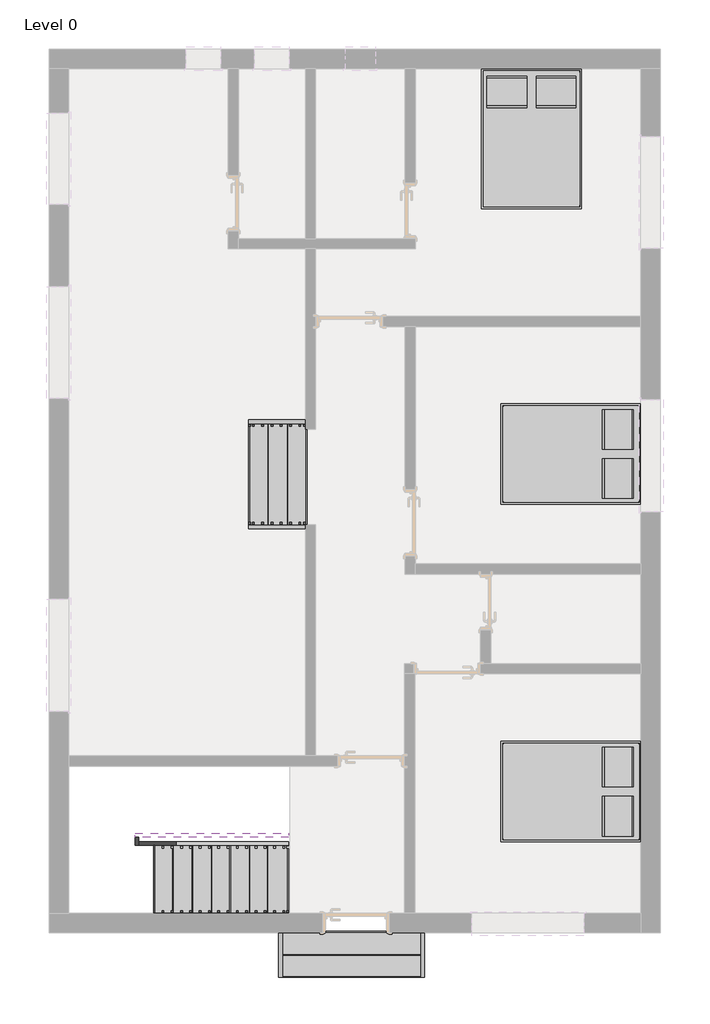
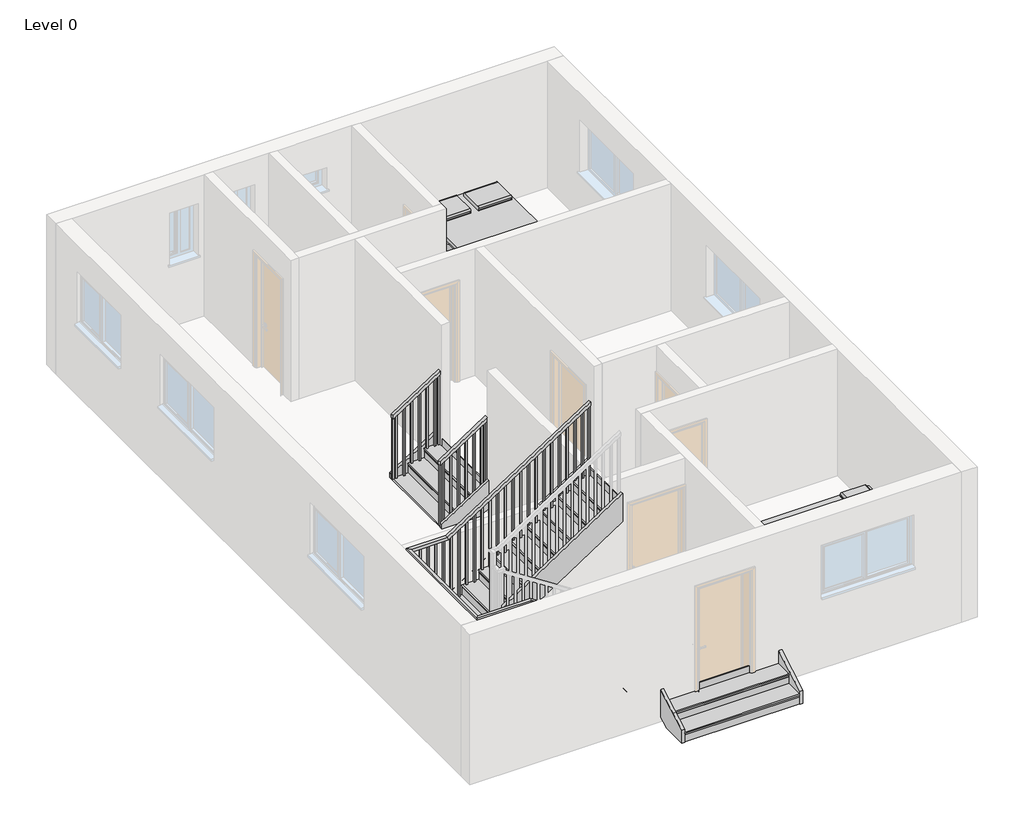
# One storey, part 2 of 2: 10 members, 3 furniture elements, 3 railings, 3 stair flights.
"""IFC4 building model written with IfcOpenShell, lengths in millimetres."""

from ifc_helpers import new_model, si_unit, frame, origin, place, context, project, spatial, polyline, outline, extrude, faceted_brep, transform, mapped, element, save
from components import furniture_bed_1_1346x1880x355mm_double_93dec6ea, wood_steps_w_50mm_tread_10mm_nosing_13mm_riser_0e3a26d2, wood_steps_w_50mm_tread_10mm_nosing_13mm_riser_e56a5079, wood_steps_w_50mm_tread_10mm_nosing_13mm_riser_d55d0cb6

model = new_model("IFC4")

# Units and contexts
model_context = context("Model", 3, world=origin())
ifc_project = project(units=[si_unit("LENGTHUNIT", "METRE", prefix="MILLI")], contexts=[model_context])

# Site, building, storey
site = spatial("IfcSite", under=ifc_project)
building = spatial("IfcBuilding", under=site)
storey = spatial("IfcBuildingStorey", under=building, Name="Level 0", Elevation=0.0)

# Furniture
placement = place(None, origin())
furniture_bed_1_1346x1880x355mm_double_shape = furniture_bed_1_1346x1880x355mm_double_93dec6ea(model_context)
element("IfcFurniture", 1, ObjectType="Furniture_Bed_1 : 1346x1880x355mm-Double", at=placement, inside=storey, context=model_context, shape_type="MappedRepresentation", body=[
    mapped(furniture_bed_1_1346x1880x355mm_double_shape, transform((-1450.4609005, 2546.998858, 400.0), x_axis=(0.0, -1.0, 0.0), y_axis=(1.0, 0.0, 0.0), z_axis=(0.0, 0.0, 1.0))),
])
element("IfcFurniture", 2, ObjectType="Furniture_Bed_1 : 1346x1880x355mm-Double", at=placement, inside=storey, context=model_context, shape_type="MappedRepresentation", body=[
    mapped(furniture_bed_1_1346x1880x355mm_double_shape, transform((-1450.4609005, 7079.151317, 400.0), x_axis=(0.0, -1.0, 0.0), y_axis=(1.0, 0.0, 0.0), z_axis=(0.0, 0.0, 1.0))),
])
element("IfcFurniture", 3, ObjectType="Furniture_Bed_1 : 1346x1880x355mm-Double", at=placement, inside=storey, context=model_context, shape_type="MappedRepresentation", body=[
    mapped(furniture_bed_1_1346x1880x355mm_double_shape, transform((-2557.0428677, 11207.1937668, 400.0), x_axis=(1.0, 0.0, 0.0), y_axis=(0.0, 1.0, 0.0), z_axis=(0.0, 0.0, 1.0))),
])

# Members
element("IfcMember", 4, ObjectType="Stringer-50mm_Width", at=placement, inside=storey, context=model_context, shape_type="SweptSolid", body=[
    extrude(outline(polyline([(230.7827164, -6016.6079187), (0.0, -6016.6079187), (0.0, -5634.3345887), (241.6372396, -5254.8904087), (715.8588519, -5254.8904087), (230.7827164, -6016.6079187)])), frame((0.0, 7148.1063074, 0.0), z_axis=(0.0, 1.0, 0.0), x_axis=(0.0, 0.0, 1.0)), (0.0, 0.0, 1.0), 50.0),
])
element("IfcMember", 5, ObjectType="Stringer-50mm_Width", at=placement, inside=storey, context=model_context, shape_type="SweptSolid", body=[
    extrude(outline(polyline([(230.7827164, -6016.6079187), (0.0, -6016.6079187), (0.0, -5634.3345887), (241.6372396, -5254.8904087), (715.8588519, -5254.8904087), (230.7827164, -6016.6079187)])), frame((0.0, 5736.998858, 0.0), z_axis=(0.0, 1.0, 0.0), x_axis=(0.0, 0.0, 1.0)), (0.0, 0.0, 1.0), 50.0),
])
element("IfcMember", 6, ObjectType="Stringer-50mm_Width", at=placement, inside=storey, context=model_context, shape_type="SweptSolid", body=[
    extrude(outline(polyline([(-287.2357414, 0.0), (-287.2357414, 221.2018083), (312.7642586, 554.5351417), (312.7642586, 96.9515798), (138.2514149, 0.0), (-287.2357414, 0.0)])), frame((-5613.3767794, 0.0, 0.0), z_axis=(1.0, 0.0, 0.0), x_axis=(0.0, 1.0, 0.0)), (0.0, 0.0, 1.0), 50.0),
])
element("IfcMember", 7, ObjectType="Stringer-50mm_Width", at=placement, inside=storey, context=model_context, shape_type="SweptSolid", body=[
    extrude(outline(polyline([(-287.2357414, 0.0), (-287.2357414, 221.2018083), (312.7642586, 554.5351417), (312.7642586, 96.9515798), (138.2514149, 0.0), (-287.2357414, 0.0)])), frame((-3703.3767794, 0.0, 0.0), z_axis=(1.0, 0.0, 0.0), x_axis=(0.0, 1.0, 0.0)), (0.0, 0.0, 1.0), 50.0),
])
element("IfcMember", 8, ObjectType="Stringer-50mm_Width", at=placement, inside=storey, context=model_context, shape_type="SweptSolid", body=[
    extrude(outline(polyline([(0.0, -5481.4951322), (214.9211649, -5481.4951322), (1542.4365081, -7506.9042559), (1542.4365081, -8236.5950487), (0.0, -5883.2776334), (0.0, -5481.4951322)])), frame((0.0, 522.7642586, 0.0), z_axis=(0.0, 1.0, 0.0), x_axis=(0.0, 0.0, 1.0)), (0.0, 0.0, 1.0), 50.0),
])
element("IfcMember", 9, ObjectType="Stringer-50mm_Width", at=placement, inside=storey, context=model_context, shape_type="SweptSolid", body=[
    extrude(outline(polyline([(-8434.8904087, 522.7642586), (-8484.8904087, 522.7642586), (-8484.8904087, 2546.998858), (-8434.8904087, 2546.998858), (-8434.8904087, 522.7642586)])), frame((0.0, 0.0, 1142.4365081), z_axis=(0.0, 0.0, 1.0), x_axis=(1.0, 0.0, 0.0)), (0.0, 0.0, 1.0), 400.0),
])
element("IfcMember", 10, ObjectType="Stringer-50mm_Width", at=placement, inside=storey, context=model_context, shape_type="SweptSolid", body=[
    extrude(outline(polyline([(1142.4365081, -7710.9666442), (2603.7006078, -5481.4951322), (3081.9623634, -5481.4951322), (1142.4365081, -8440.657437), (1142.4365081, -7710.9666442)])), frame((0.0, 2546.998858, 0.0), z_axis=(0.0, 1.0, 0.0), x_axis=(0.0, 0.0, 1.0)), (0.0, 0.0, 1.0), 50.0),
])
element("IfcMember", 11, ObjectType="Stringer-50mm_Width", at=placement, inside=storey, context=model_context, shape_type="SweptSolid", body=[
    extrude(outline(polyline([(0.0, -5481.4951322), (214.9211649, -5481.4951322), (1532.3368952, -7491.4951322), (1054.0751396, -7491.4951322), (0.0, -5883.2776334), (0.0, -5481.4951322)])), frame((0.0, 1486.5182736, 0.0), z_axis=(0.0, 1.0, 0.0), x_axis=(0.0, 0.0, 1.0)), (0.0, 0.0, 1.0), 50.0),
])
element("IfcMember", 12, ObjectType="Stringer-50mm_Width", at=placement, inside=storey, context=model_context, shape_type="SweptSolid", body=[
    extrude(outline(polyline([(-7491.4951322, 1486.5182736), (-7541.4951322, 1486.5182736), (-7541.4951322, 1596.5182736), (-7491.4951322, 1596.5182736), (-7491.4951322, 1486.5182736)])), frame((0.0, 0.0, 1142.4365081), z_axis=(0.0, 0.0, 1.0), x_axis=(1.0, 0.0, 0.0)), (0.0, 0.0, 1.0), 400.0),
])
element("IfcMember", 13, ObjectType="Stringer-50mm_Width", at=placement, inside=storey, context=model_context, shape_type="SweptSolid", body=[
    extrude(outline(polyline([(1731.7750974, -7541.4951322), (1253.5133419, -7541.4951322), (2603.7006078, -5481.4951322), (3081.9623634, -5481.4951322), (1731.7750974, -7541.4951322)])), frame((0.0, 1596.5182736, 0.0), z_axis=(0.0, 1.0, 0.0), x_axis=(0.0, 0.0, 1.0)), (0.0, 0.0, 1.0), 50.0),
])

# Railings
element("IfcRailing", 14, ObjectType="1100mm", at=placement, inside=storey, context=model_context, shape_type="SweptSolid", body=[
    extrude(outline(polyline([(1266.6666667, -6016.6079187), (1206.8570557, -6016.6079187), (1706.8570557, -5254.8904087), (1766.6666667, -5254.8904087), (1266.6666667, -6016.6079187)])), frame((0.0, 5787.398858, 0.0), z_axis=(0.0, 1.0, 0.0), x_axis=(0.0, 0.0, 1.0)), (0.0, 0.0, 1.0), 50.0),
    extrude(outline(polyline([(1649.9347, -5341.6079187), (500.0, -5341.6079187), (500.0, -5316.6079187), (1666.3449832, -5316.6079187), (1649.9347, -5341.6079187)])), frame((0.0, 5799.898858, 0.0), z_axis=(0.0, 1.0, 0.0), x_axis=(0.0, 0.0, 1.0)), (0.0, 0.0, 1.0), 25.0),
    extrude(outline(polyline([(1567.8832844, -5466.6079187), (500.0, -5466.6079187), (500.0, -5441.6079187), (1584.2935675, -5441.6079187), (1567.8832844, -5466.6079187)])), frame((0.0, 5799.898858, 0.0), z_axis=(0.0, 1.0, 0.0), x_axis=(0.0, 0.0, 1.0)), (0.0, 0.0, 1.0), 25.0),
    extrude(outline(polyline([(1485.8318688, -5591.6079187), (333.3333333, -5591.6079187), (333.3333333, -5566.6079187), (1502.2421519, -5566.6079187), (1485.8318688, -5591.6079187)])), frame((0.0, 5799.898858, 0.0), z_axis=(0.0, 1.0, 0.0), x_axis=(0.0, 0.0, 1.0)), (0.0, 0.0, 1.0), 25.0),
    extrude(outline(polyline([(1403.7804532, -5716.6079187), (333.3333333, -5716.6079187), (333.3333333, -5691.6079187), (1420.1907363, -5691.6079187), (1403.7804532, -5716.6079187)])), frame((0.0, 5799.898858, 0.0), z_axis=(0.0, 1.0, 0.0), x_axis=(0.0, 0.0, 1.0)), (0.0, 0.0, 1.0), 25.0),
    extrude(outline(polyline([(1321.7290375, -5841.6079187), (166.6666667, -5841.6079187), (166.6666667, -5816.6079187), (1338.1393207, -5816.6079187), (1321.7290375, -5841.6079187)])), frame((0.0, 5799.898858, 0.0), z_axis=(0.0, 1.0, 0.0), x_axis=(0.0, 0.0, 1.0)), (0.0, 0.0, 1.0), 25.0),
    extrude(outline(polyline([(1239.6776219, -5966.6079187), (166.6666667, -5966.6079187), (166.6666667, -5941.6079187), (1256.087905, -5941.6079187), (1239.6776219, -5966.6079187)])), frame((0.0, 5799.898858, 0.0), z_axis=(0.0, 1.0, 0.0), x_axis=(0.0, 0.0, 1.0)), (0.0, 0.0, 1.0), 25.0),
    extrude(outline(polyline([(1690.4467725, -5279.8904087), (500.0, -5279.8904087), (500.0, -5254.8904087), (1706.8570557, -5254.8904087), (1690.4467725, -5279.8904087)])), frame((0.0, 5799.898858, 0.0), z_axis=(0.0, 1.0, 0.0), x_axis=(0.0, 0.0, 1.0)), (0.0, 0.0, 1.0), 25.0),
    extrude(outline(polyline([(1206.8570557, -6016.6079187), (166.6666667, -6016.6079187), (166.6666667, -5991.6079187), (1223.2673388, -5991.6079187), (1206.8570557, -6016.6079187)])), frame((0.0, 5799.898858, 0.0), z_axis=(0.0, 1.0, 0.0), x_axis=(0.0, 0.0, 1.0)), (0.0, 0.0, 1.0), 25.0),
])
element("IfcRailing", 15, ObjectType="1100mm", at=placement, inside=storey, context=model_context, shape_type="SweptSolid", body=[
    extrude(outline(polyline([(1266.6666667, -6016.6079187), (1206.8570557, -6016.6079187), (1706.8570557, -5254.8904087), (1766.6666667, -5254.8904087), (1266.6666667, -6016.6079187)])), frame((0.0, 7097.7063074, 0.0), z_axis=(0.0, 1.0, 0.0), x_axis=(0.0, 0.0, 1.0)), (0.0, 0.0, 1.0), 50.0),
    extrude(outline(polyline([(500.0, -5341.6079187), (500.0, -5316.6079187), (1666.3449832, -5316.6079187), (1649.9347, -5341.6079187), (500.0, -5341.6079187)])), frame((0.0, 7110.2063074, 0.0), z_axis=(0.0, 1.0, 0.0), x_axis=(0.0, 0.0, 1.0)), (0.0, 0.0, 1.0), 25.0),
    extrude(outline(polyline([(500.0, -5466.6079187), (500.0, -5441.6079187), (1584.2935675, -5441.6079187), (1567.8832844, -5466.6079187), (500.0, -5466.6079187)])), frame((0.0, 7110.2063074, 0.0), z_axis=(0.0, 1.0, 0.0), x_axis=(0.0, 0.0, 1.0)), (0.0, 0.0, 1.0), 25.0),
    extrude(outline(polyline([(333.3333333, -5591.6079187), (333.3333333, -5566.6079187), (1502.2421519, -5566.6079187), (1485.8318688, -5591.6079187), (333.3333333, -5591.6079187)])), frame((0.0, 7110.2063074, 0.0), z_axis=(0.0, 1.0, 0.0), x_axis=(0.0, 0.0, 1.0)), (0.0, 0.0, 1.0), 25.0),
    extrude(outline(polyline([(333.3333333, -5716.6079187), (333.3333333, -5691.6079187), (1420.1907363, -5691.6079187), (1403.7804532, -5716.6079187), (333.3333333, -5716.6079187)])), frame((0.0, 7110.2063074, 0.0), z_axis=(0.0, 1.0, 0.0), x_axis=(0.0, 0.0, 1.0)), (0.0, 0.0, 1.0), 25.0),
    extrude(outline(polyline([(166.6666667, -5841.6079187), (166.6666667, -5816.6079187), (1338.1393207, -5816.6079187), (1321.7290375, -5841.6079187), (166.6666667, -5841.6079187)])), frame((0.0, 7110.2063074, 0.0), z_axis=(0.0, 1.0, 0.0), x_axis=(0.0, 0.0, 1.0)), (0.0, 0.0, 1.0), 25.0),
    extrude(outline(polyline([(166.6666667, -5966.6079187), (166.6666667, -5941.6079187), (1256.087905, -5941.6079187), (1239.6776219, -5966.6079187), (166.6666667, -5966.6079187)])), frame((0.0, 7110.2063074, 0.0), z_axis=(0.0, 1.0, 0.0), x_axis=(0.0, 0.0, 1.0)), (0.0, 0.0, 1.0), 25.0),
    extrude(outline(polyline([(500.0, -5279.8904087), (500.0, -5254.8904087), (1706.8570557, -5254.8904087), (1690.4467725, -5279.8904087), (500.0, -5279.8904087)])), frame((0.0, 7110.2063074, 0.0), z_axis=(0.0, 1.0, 0.0), x_axis=(0.0, 0.0, 1.0)), (0.0, 0.0, 1.0), 25.0),
    extrude(outline(polyline([(166.6666667, -6016.6079187), (166.6666667, -5991.6079187), (1223.2673388, -5991.6079187), (1206.8570557, -6016.6079187), (166.6666667, -6016.6079187)])), frame((0.0, 7110.2063074, 0.0), z_axis=(0.0, 1.0, 0.0), x_axis=(0.0, 0.0, 1.0)), (0.0, 0.0, 1.0), 25.0),
])
element("IfcRailing", 16, ObjectType="1100mm", at=placement, inside=storey, context=model_context, shape_type="SolidModel", body=[
    faceted_brep([(-5481.4951322, 573.1642586, 1266.6666667), (-5481.4951322, 573.1642586, 1207.1072108), (-5481.4951322, 623.1642586, 1207.1072108), (-5481.4951322, 623.1642586, 1266.6666667), (-7541.4951322, 573.1642586, 2600.0), (-7556.2644916, 573.1642586, 2550.0), (-7556.2644916, 623.1642586, 2550.0), (-7541.4951322, 623.1642586, 2600.0), (-8434.4904087, 573.1642586, 2600.0), (-8434.4904087, 573.1642586, 2550.0), (-8384.4904087, 623.1642586, 2550.0), (-8384.4904087, 623.1642586, 2600.0), (-8434.4904087, 2546.598858, 2600.0), (-8434.4904087, 2546.598858, 2550.0), (-8384.4904087, 2496.598858, 2550.0), (-8384.4904087, 2496.598858, 2600.0), (-7798.9951322, 2546.598858, 2600.0), (-7784.2257728, 2546.598858, 2550.0), (-7784.2257728, 2496.598858, 2550.0), (-7798.9951322, 2496.598858, 2600.0), (-5481.4951322, 2546.598858, 4100.0), (-5481.4951322, 2496.598858, 4100.0), (-5481.4951322, 2496.598858, 4040.4405441), (-5481.4951322, 2546.598858, 4040.4405441)], [[[0, 1, 2, 3]], [[1, 0, 4, 5]], [[2, 1, 5, 6]], [[3, 2, 6, 7]], [[0, 3, 7, 4]], [[5, 4, 8, 9]], [[6, 5, 9, 10]], [[7, 6, 10, 11]], [[4, 7, 11, 8]], [[9, 8, 12, 13]], [[10, 9, 13, 14]], [[11, 10, 14, 15]], [[8, 11, 15, 12]], [[13, 12, 16, 17]], [[14, 13, 17, 18]], [[15, 14, 18, 19]], [[12, 15, 19, 16]], [[20, 21, 22, 23]], [[17, 16, 20, 23]], [[18, 17, 23, 22]], [[19, 18, 22, 21]], [[16, 19, 21, 20]]]),
    extrude(outline(polyline([(2833.3333333, -5609.4904087), (2833.3333333, -5584.4904087), (3973.7769347, -5584.4904087), (3957.5957049, -5609.4904087), (2833.3333333, -5609.4904087)])), frame((0.0, 2509.098858, 0.0), z_axis=(0.0, 1.0, 0.0), x_axis=(0.0, 0.0, 1.0)), (0.0, 0.0, 1.0), 25.0),
    extrude(outline(polyline([(2833.3333333, -5734.4904087), (2833.3333333, -5709.4904087), (3892.8707858, -5709.4904087), (3876.689556, -5734.4904087), (2833.3333333, -5734.4904087)])), frame((0.0, 2509.098858, 0.0), z_axis=(0.0, 1.0, 0.0), x_axis=(0.0, 0.0, 1.0)), (0.0, 0.0, 1.0), 25.0),
    extrude(outline(polyline([(2666.6666667, -5859.4904087), (2666.6666667, -5834.4904087), (3811.964637, -5834.4904087), (3795.7834072, -5859.4904087), (2666.6666667, -5859.4904087)])), frame((0.0, 2509.098858, 0.0), z_axis=(0.0, 1.0, 0.0), x_axis=(0.0, 0.0, 1.0)), (0.0, 0.0, 1.0), 25.0),
    extrude(outline(polyline([(2666.6666667, -5984.4904087), (2666.6666667, -5959.4904087), (3731.0584881, -5959.4904087), (3714.8772583, -5984.4904087), (2666.6666667, -5984.4904087)])), frame((0.0, 2509.098858, 0.0), z_axis=(0.0, 1.0, 0.0), x_axis=(0.0, 0.0, 1.0)), (0.0, 0.0, 1.0), 25.0),
    extrude(outline(polyline([(2500.0, -6109.4904087), (2500.0, -6084.4904087), (3650.1523392, -6084.4904087), (3633.9711094, -6109.4904087), (2500.0, -6109.4904087)])), frame((0.0, 2509.098858, 0.0), z_axis=(0.0, 1.0, 0.0), x_axis=(0.0, 0.0, 1.0)), (0.0, 0.0, 1.0), 25.0),
    extrude(outline(polyline([(2500.0, -6234.4904087), (2500.0, -6209.4904087), (3569.2461904, -6209.4904087), (3553.0649606, -6234.4904087), (2500.0, -6234.4904087)])), frame((0.0, 2509.098858, 0.0), z_axis=(0.0, 1.0, 0.0), x_axis=(0.0, 0.0, 1.0)), (0.0, 0.0, 1.0), 25.0),
    extrude(outline(polyline([(2333.3333333, -6359.4904087), (2333.3333333, -6334.4904087), (3488.3400415, -6334.4904087), (3472.1588117, -6359.4904087), (2333.3333333, -6359.4904087)])), frame((0.0, 2509.098858, 0.0), z_axis=(0.0, 1.0, 0.0), x_axis=(0.0, 0.0, 1.0)), (0.0, 0.0, 1.0), 25.0),
    extrude(outline(polyline([(2333.3333333, -6484.4904087), (2333.3333333, -6459.4904087), (3407.4338926, -6459.4904087), (3391.2526628, -6484.4904087), (2333.3333333, -6484.4904087)])), frame((0.0, 2509.098858, 0.0), z_axis=(0.0, 1.0, 0.0), x_axis=(0.0, 0.0, 1.0)), (0.0, 0.0, 1.0), 25.0),
    extrude(outline(polyline([(2166.6666667, -6609.4904087), (2166.6666667, -6584.4904087), (3326.5277438, -6584.4904087), (3310.346514, -6609.4904087), (2166.6666667, -6609.4904087)])), frame((0.0, 2509.098858, 0.0), z_axis=(0.0, 1.0, 0.0), x_axis=(0.0, 0.0, 1.0)), (0.0, 0.0, 1.0), 25.0),
    extrude(outline(polyline([(2166.6666667, -6734.4904087), (2166.6666667, -6709.4904087), (3245.6215949, -6709.4904087), (3229.4403651, -6734.4904087), (2166.6666667, -6734.4904087)])), frame((0.0, 2509.098858, 0.0), z_axis=(0.0, 1.0, 0.0), x_axis=(0.0, 0.0, 1.0)), (0.0, 0.0, 1.0), 25.0),
    extrude(outline(polyline([(2000.0, -6859.4904087), (2000.0, -6834.4904087), (3164.715446, -6834.4904087), (3148.5342162, -6859.4904087), (2000.0, -6859.4904087)])), frame((0.0, 2509.098858, 0.0), z_axis=(0.0, 1.0, 0.0), x_axis=(0.0, 0.0, 1.0)), (0.0, 0.0, 1.0), 25.0),
    extrude(outline(polyline([(2000.0, -6984.4904087), (2000.0, -6959.4904087), (3083.8092971, -6959.4904087), (3067.6280674, -6984.4904087), (2000.0, -6984.4904087)])), frame((0.0, 2509.098858, 0.0), z_axis=(0.0, 1.0, 0.0), x_axis=(0.0, 0.0, 1.0)), (0.0, 0.0, 1.0), 25.0),
    extrude(outline(polyline([(1833.3333333, -7109.4904087), (1833.3333333, -7084.4904087), (3002.9031483, -7084.4904087), (2986.7219185, -7109.4904087), (1833.3333333, -7109.4904087)])), frame((0.0, 2509.098858, 0.0), z_axis=(0.0, 1.0, 0.0), x_axis=(0.0, 0.0, 1.0)), (0.0, 0.0, 1.0), 25.0),
    extrude(outline(polyline([(1833.3333333, -7234.4904087), (1833.3333333, -7209.4904087), (2921.9969994, -7209.4904087), (2905.8157696, -7234.4904087), (1833.3333333, -7234.4904087)])), frame((0.0, 2509.098858, 0.0), z_axis=(0.0, 1.0, 0.0), x_axis=(0.0, 0.0, 1.0)), (0.0, 0.0, 1.0), 25.0),
    extrude(outline(polyline([(1666.6666667, -7359.4904087), (1666.6666667, -7334.4904087), (2841.0908505, -7334.4904087), (2824.9096208, -7359.4904087), (1666.6666667, -7359.4904087)])), frame((0.0, 2509.098858, 0.0), z_axis=(0.0, 1.0, 0.0), x_axis=(0.0, 0.0, 1.0)), (0.0, 0.0, 1.0), 25.0),
    extrude(outline(polyline([(1666.6666667, -7484.4904087), (1666.6666667, -7459.4904087), (2760.1847017, -7459.4904087), (2744.0034719, -7484.4904087), (1666.6666667, -7484.4904087)])), frame((0.0, 2509.098858, 0.0), z_axis=(0.0, 1.0, 0.0), x_axis=(0.0, 0.0, 1.0)), (0.0, 0.0, 1.0), 25.0),
    extrude(outline(polyline([(1500.0, -7609.4904087), (1500.0, -7584.4904087), (2679.2785528, -7584.4904087), (2663.097323, -7609.4904087), (1500.0, -7609.4904087)])), frame((0.0, 2509.098858, 0.0), z_axis=(0.0, 1.0, 0.0), x_axis=(0.0, 0.0, 1.0)), (0.0, 0.0, 1.0), 25.0),
    extrude(outline(polyline([(1500.0, -7734.4904087), (1500.0, -7709.4904087), (2598.3724039, -7709.4904087), (2582.1911742, -7734.4904087), (1500.0, -7734.4904087)])), frame((0.0, 2509.098858, 0.0), z_axis=(0.0, 1.0, 0.0), x_axis=(0.0, 0.0, 1.0)), (0.0, 0.0, 1.0), 25.0),
    extrude(outline(polyline([(-7859.4904087, 2534.098858), (-7834.4904087, 2534.098858), (-7834.4904087, 2509.098858), (-7859.4904087, 2509.098858), (-7859.4904087, 2534.098858)])), frame((0.0, 0.0, 1500.0), z_axis=(0.0, 0.0, 1.0), x_axis=(1.0, 0.0, 0.0)), (0.0, 0.0, 1.0), 1050.0),
    extrude(outline(polyline([(-7984.4904087, 2534.098858), (-7959.4904087, 2534.098858), (-7959.4904087, 2509.098858), (-7984.4904087, 2509.098858), (-7984.4904087, 2534.098858)])), frame((0.0, 0.0, 1500.0), z_axis=(0.0, 0.0, 1.0), x_axis=(1.0, 0.0, 0.0)), (0.0, 0.0, 1.0), 1050.0),
    extrude(outline(polyline([(-8109.4904087, 2534.098858), (-8084.4904087, 2534.098858), (-8084.4904087, 2509.098858), (-8109.4904087, 2509.098858), (-8109.4904087, 2534.098858)])), frame((0.0, 0.0, 1500.0), z_axis=(0.0, 0.0, 1.0), x_axis=(1.0, 0.0, 0.0)), (0.0, 0.0, 1.0), 1050.0),
    extrude(outline(polyline([(-8234.4904087, 2534.098858), (-8209.4904087, 2534.098858), (-8209.4904087, 2509.098858), (-8234.4904087, 2509.098858), (-8234.4904087, 2534.098858)])), frame((0.0, 0.0, 1500.0), z_axis=(0.0, 0.0, 1.0), x_axis=(1.0, 0.0, 0.0)), (0.0, 0.0, 1.0), 1050.0),
    extrude(outline(polyline([(-8359.4904087, 2534.098858), (-8334.4904087, 2534.098858), (-8334.4904087, 2509.098858), (-8359.4904087, 2509.098858), (-8359.4904087, 2534.098858)])), frame((0.0, 0.0, 1500.0), z_axis=(0.0, 0.0, 1.0), x_axis=(1.0, 0.0, 0.0)), (0.0, 0.0, 1.0), 1050.0),
    extrude(outline(polyline([(-8421.9904087, 2398.1642586), (-8421.9904087, 2423.1642586), (-8396.9904087, 2423.1642586), (-8396.9904087, 2398.1642586), (-8421.9904087, 2398.1642586)])), frame((0.0, 0.0, 1500.0), z_axis=(0.0, 0.0, 1.0), x_axis=(1.0, 0.0, 0.0)), (0.0, 0.0, 1.0), 1050.0),
    extrude(outline(polyline([(-8421.9904087, 2273.1642586), (-8421.9904087, 2298.1642586), (-8396.9904087, 2298.1642586), (-8396.9904087, 2273.1642586), (-8421.9904087, 2273.1642586)])), frame((0.0, 0.0, 1500.0), z_axis=(0.0, 0.0, 1.0), x_axis=(1.0, 0.0, 0.0)), (0.0, 0.0, 1.0), 1050.0),
    extrude(outline(polyline([(-8421.9904087, 2148.1642586), (-8421.9904087, 2173.1642586), (-8396.9904087, 2173.1642586), (-8396.9904087, 2148.1642586), (-8421.9904087, 2148.1642586)])), frame((0.0, 0.0, 1500.0), z_axis=(0.0, 0.0, 1.0), x_axis=(1.0, 0.0, 0.0)), (0.0, 0.0, 1.0), 1050.0),
    extrude(outline(polyline([(-8421.9904087, 2023.1642586), (-8421.9904087, 2048.1642586), (-8396.9904087, 2048.1642586), (-8396.9904087, 2023.1642586), (-8421.9904087, 2023.1642586)])), frame((0.0, 0.0, 1500.0), z_axis=(0.0, 0.0, 1.0), x_axis=(1.0, 0.0, 0.0)), (0.0, 0.0, 1.0), 1050.0),
    extrude(outline(polyline([(-8421.9904087, 1898.1642586), (-8421.9904087, 1923.1642586), (-8396.9904087, 1923.1642586), (-8396.9904087, 1898.1642586), (-8421.9904087, 1898.1642586)])), frame((0.0, 0.0, 1500.0), z_axis=(0.0, 0.0, 1.0), x_axis=(1.0, 0.0, 0.0)), (0.0, 0.0, 1.0), 1050.0),
    extrude(outline(polyline([(-8421.9904087, 1773.1642586), (-8421.9904087, 1798.1642586), (-8396.9904087, 1798.1642586), (-8396.9904087, 1773.1642586), (-8421.9904087, 1773.1642586)])), frame((0.0, 0.0, 1500.0), z_axis=(0.0, 0.0, 1.0), x_axis=(1.0, 0.0, 0.0)), (0.0, 0.0, 1.0), 1050.0),
    extrude(outline(polyline([(-8421.9904087, 1648.1642586), (-8421.9904087, 1673.1642586), (-8396.9904087, 1673.1642586), (-8396.9904087, 1648.1642586), (-8421.9904087, 1648.1642586)])), frame((0.0, 0.0, 1500.0), z_axis=(0.0, 0.0, 1.0), x_axis=(1.0, 0.0, 0.0)), (0.0, 0.0, 1.0), 1050.0),
    extrude(outline(polyline([(-8421.9904087, 1523.1642586), (-8421.9904087, 1548.1642586), (-8396.9904087, 1548.1642586), (-8396.9904087, 1523.1642586), (-8421.9904087, 1523.1642586)])), frame((0.0, 0.0, 1500.0), z_axis=(0.0, 0.0, 1.0), x_axis=(1.0, 0.0, 0.0)), (0.0, 0.0, 1.0), 1050.0),
    extrude(outline(polyline([(-8421.9904087, 1398.1642586), (-8421.9904087, 1423.1642586), (-8396.9904087, 1423.1642586), (-8396.9904087, 1398.1642586), (-8421.9904087, 1398.1642586)])), frame((0.0, 0.0, 1500.0), z_axis=(0.0, 0.0, 1.0), x_axis=(1.0, 0.0, 0.0)), (0.0, 0.0, 1.0), 1050.0),
    extrude(outline(polyline([(-8421.9904087, 1273.1642586), (-8421.9904087, 1298.1642586), (-8396.9904087, 1298.1642586), (-8396.9904087, 1273.1642586), (-8421.9904087, 1273.1642586)])), frame((0.0, 0.0, 1500.0), z_axis=(0.0, 0.0, 1.0), x_axis=(1.0, 0.0, 0.0)), (0.0, 0.0, 1.0), 1050.0),
    extrude(outline(polyline([(-8421.9904087, 1148.1642586), (-8421.9904087, 1173.1642586), (-8396.9904087, 1173.1642586), (-8396.9904087, 1148.1642586), (-8421.9904087, 1148.1642586)])), frame((0.0, 0.0, 1500.0), z_axis=(0.0, 0.0, 1.0), x_axis=(1.0, 0.0, 0.0)), (0.0, 0.0, 1.0), 1050.0),
    extrude(outline(polyline([(-8421.9904087, 1023.1642586), (-8421.9904087, 1048.1642586), (-8396.9904087, 1048.1642586), (-8396.9904087, 1023.1642586), (-8421.9904087, 1023.1642586)])), frame((0.0, 0.0, 1500.0), z_axis=(0.0, 0.0, 1.0), x_axis=(1.0, 0.0, 0.0)), (0.0, 0.0, 1.0), 1050.0),
    extrude(outline(polyline([(-8421.9904087, 898.1642586), (-8421.9904087, 923.1642586), (-8396.9904087, 923.1642586), (-8396.9904087, 898.1642586), (-8421.9904087, 898.1642586)])), frame((0.0, 0.0, 1500.0), z_axis=(0.0, 0.0, 1.0), x_axis=(1.0, 0.0, 0.0)), (0.0, 0.0, 1.0), 1050.0),
    extrude(outline(polyline([(-8421.9904087, 773.1642586), (-8421.9904087, 798.1642586), (-8396.9904087, 798.1642586), (-8396.9904087, 773.1642586), (-8421.9904087, 773.1642586)])), frame((0.0, 0.0, 1500.0), z_axis=(0.0, 0.0, 1.0), x_axis=(1.0, 0.0, 0.0)), (0.0, 0.0, 1.0), 1050.0),
    extrude(outline(polyline([(-8421.9904087, 648.1642586), (-8421.9904087, 673.1642586), (-8396.9904087, 673.1642586), (-8396.9904087, 648.1642586), (-8421.9904087, 648.1642586)])), frame((0.0, 0.0, 1500.0), z_axis=(0.0, 0.0, 1.0), x_axis=(1.0, 0.0, 0.0)), (0.0, 0.0, 1.0), 1050.0),
    extrude(outline(polyline([(-8281.4951322, 585.6642586), (-8306.4951322, 585.6642586), (-8306.4951322, 610.6642586), (-8281.4951322, 610.6642586), (-8281.4951322, 585.6642586)])), frame((0.0, 0.0, 1500.0), z_axis=(0.0, 0.0, 1.0), x_axis=(1.0, 0.0, 0.0)), (0.0, 0.0, 1.0), 1050.0),
    extrude(outline(polyline([(-8156.4951322, 585.6642586), (-8181.4951322, 585.6642586), (-8181.4951322, 610.6642586), (-8156.4951322, 610.6642586), (-8156.4951322, 585.6642586)])), frame((0.0, 0.0, 1500.0), z_axis=(0.0, 0.0, 1.0), x_axis=(1.0, 0.0, 0.0)), (0.0, 0.0, 1.0), 1050.0),
    extrude(outline(polyline([(-8031.4951322, 585.6642586), (-8056.4951322, 585.6642586), (-8056.4951322, 610.6642586), (-8031.4951322, 610.6642586), (-8031.4951322, 585.6642586)])), frame((0.0, 0.0, 1500.0), z_axis=(0.0, 0.0, 1.0), x_axis=(1.0, 0.0, 0.0)), (0.0, 0.0, 1.0), 1050.0),
    extrude(outline(polyline([(-7906.4951322, 585.6642586), (-7931.4951322, 585.6642586), (-7931.4951322, 610.6642586), (-7906.4951322, 610.6642586), (-7906.4951322, 585.6642586)])), frame((0.0, 0.0, 1500.0), z_axis=(0.0, 0.0, 1.0), x_axis=(1.0, 0.0, 0.0)), (0.0, 0.0, 1.0), 1050.0),
    extrude(outline(polyline([(-7781.4951322, 585.6642586), (-7806.4951322, 585.6642586), (-7806.4951322, 610.6642586), (-7781.4951322, 610.6642586), (-7781.4951322, 585.6642586)])), frame((0.0, 0.0, 1500.0), z_axis=(0.0, 0.0, 1.0), x_axis=(1.0, 0.0, 0.0)), (0.0, 0.0, 1.0), 1050.0),
    extrude(outline(polyline([(-7656.4951322, 585.6642586), (-7681.4951322, 585.6642586), (-7681.4951322, 610.6642586), (-7656.4951322, 610.6642586), (-7656.4951322, 585.6642586)])), frame((0.0, 0.0, 1500.0), z_axis=(0.0, 0.0, 1.0), x_axis=(1.0, 0.0, 0.0)), (0.0, 0.0, 1.0), 1050.0),
    extrude(outline(polyline([(-7531.4951322, 585.6642586), (-7556.4951322, 585.6642586), (-7556.4951322, 610.6642586), (-7531.4951322, 610.6642586), (-7531.4951322, 585.6642586)])), frame((0.0, 0.0, 1500.0), z_axis=(0.0, 0.0, 1.0), x_axis=(1.0, 0.0, 0.0)), (0.0, 0.0, 1.0), 1050.0),
    extrude(outline(polyline([(2453.0619033, -7406.4951322), (2469.2431331, -7431.4951322), (1333.3333333, -7431.4951322), (1333.3333333, -7406.4951322), (2453.0619033, -7406.4951322)])), frame((0.0, 585.6642586, 0.0), z_axis=(0.0, 1.0, 0.0), x_axis=(0.0, 0.0, 1.0)), (0.0, 0.0, 1.0), 25.0),
    extrude(outline(polyline([(2372.1557544, -7281.4951322), (2388.3369842, -7306.4951322), (1333.3333333, -7306.4951322), (1333.3333333, -7281.4951322), (2372.1557544, -7281.4951322)])), frame((0.0, 585.6642586, 0.0), z_axis=(0.0, 1.0, 0.0), x_axis=(0.0, 0.0, 1.0)), (0.0, 0.0, 1.0), 25.0),
    extrude(outline(polyline([(2291.2496056, -7156.4951322), (2307.4308354, -7181.4951322), (1166.6666667, -7181.4951322), (1166.6666667, -7156.4951322), (2291.2496056, -7156.4951322)])), frame((0.0, 585.6642586, 0.0), z_axis=(0.0, 1.0, 0.0), x_axis=(0.0, 0.0, 1.0)), (0.0, 0.0, 1.0), 25.0),
    extrude(outline(polyline([(2210.3434567, -7031.4951322), (2226.5246865, -7056.4951322), (1166.6666667, -7056.4951322), (1166.6666667, -7031.4951322), (2210.3434567, -7031.4951322)])), frame((0.0, 585.6642586, 0.0), z_axis=(0.0, 1.0, 0.0), x_axis=(0.0, 0.0, 1.0)), (0.0, 0.0, 1.0), 25.0),
    extrude(outline(polyline([(2129.4373078, -6906.4951322), (2145.6185376, -6931.4951322), (1000.0, -6931.4951322), (1000.0, -6906.4951322), (2129.4373078, -6906.4951322)])), frame((0.0, 585.6642586, 0.0), z_axis=(0.0, 1.0, 0.0), x_axis=(0.0, 0.0, 1.0)), (0.0, 0.0, 1.0), 25.0),
    extrude(outline(polyline([(2048.531159, -6781.4951322), (2064.7123888, -6806.4951322), (1000.0, -6806.4951322), (1000.0, -6781.4951322), (2048.531159, -6781.4951322)])), frame((0.0, 585.6642586, 0.0), z_axis=(0.0, 1.0, 0.0), x_axis=(0.0, 0.0, 1.0)), (0.0, 0.0, 1.0), 25.0),
    extrude(outline(polyline([(1967.6250101, -6656.4951322), (1983.8062399, -6681.4951322), (833.3333333, -6681.4951322), (833.3333333, -6656.4951322), (1967.6250101, -6656.4951322)])), frame((0.0, 585.6642586, 0.0), z_axis=(0.0, 1.0, 0.0), x_axis=(0.0, 0.0, 1.0)), (0.0, 0.0, 1.0), 25.0),
    extrude(outline(polyline([(1886.7188612, -6531.4951322), (1902.900091, -6556.4951322), (833.3333333, -6556.4951322), (833.3333333, -6531.4951322), (1886.7188612, -6531.4951322)])), frame((0.0, 585.6642586, 0.0), z_axis=(0.0, 1.0, 0.0), x_axis=(0.0, 0.0, 1.0)), (0.0, 0.0, 1.0), 25.0),
    extrude(outline(polyline([(1805.8127124, -6406.4951322), (1821.9939422, -6431.4951322), (666.6666667, -6431.4951322), (666.6666667, -6406.4951322), (1805.8127124, -6406.4951322)])), frame((0.0, 585.6642586, 0.0), z_axis=(0.0, 1.0, 0.0), x_axis=(0.0, 0.0, 1.0)), (0.0, 0.0, 1.0), 25.0),
    extrude(outline(polyline([(1724.9065635, -6281.4951322), (1741.0877933, -6306.4951322), (666.6666667, -6306.4951322), (666.6666667, -6281.4951322), (1724.9065635, -6281.4951322)])), frame((0.0, 585.6642586, 0.0), z_axis=(0.0, 1.0, 0.0), x_axis=(0.0, 0.0, 1.0)), (0.0, 0.0, 1.0), 25.0),
    extrude(outline(polyline([(1644.0004146, -6156.4951322), (1660.1816444, -6181.4951322), (500.0, -6181.4951322), (500.0, -6156.4951322), (1644.0004146, -6156.4951322)])), frame((0.0, 585.6642586, 0.0), z_axis=(0.0, 1.0, 0.0), x_axis=(0.0, 0.0, 1.0)), (0.0, 0.0, 1.0), 25.0),
    extrude(outline(polyline([(1563.0942658, -6031.4951322), (1579.2754955, -6056.4951322), (500.0, -6056.4951322), (500.0, -6031.4951322), (1563.0942658, -6031.4951322)])), frame((0.0, 585.6642586, 0.0), z_axis=(0.0, 1.0, 0.0), x_axis=(0.0, 0.0, 1.0)), (0.0, 0.0, 1.0), 25.0),
    extrude(outline(polyline([(1482.1881169, -5906.4951322), (1498.3693467, -5931.4951322), (333.3333333, -5931.4951322), (333.3333333, -5906.4951322), (1482.1881169, -5906.4951322)])), frame((0.0, 585.6642586, 0.0), z_axis=(0.0, 1.0, 0.0), x_axis=(0.0, 0.0, 1.0)), (0.0, 0.0, 1.0), 25.0),
    extrude(outline(polyline([(1401.281968, -5781.4951322), (1417.4631978, -5806.4951322), (333.3333333, -5806.4951322), (333.3333333, -5781.4951322), (1401.281968, -5781.4951322)])), frame((0.0, 585.6642586, 0.0), z_axis=(0.0, 1.0, 0.0), x_axis=(0.0, 0.0, 1.0)), (0.0, 0.0, 1.0), 25.0),
    extrude(outline(polyline([(1320.3758192, -5656.4951322), (1336.5570489, -5681.4951322), (166.6666667, -5681.4951322), (166.6666667, -5656.4951322), (1320.3758192, -5656.4951322)])), frame((0.0, 585.6642586, 0.0), z_axis=(0.0, 1.0, 0.0), x_axis=(0.0, 0.0, 1.0)), (0.0, 0.0, 1.0), 25.0),
    extrude(outline(polyline([(1239.4696703, -5531.4951322), (1255.6509001, -5556.4951322), (166.6666667, -5556.4951322), (166.6666667, -5531.4951322), (1239.4696703, -5531.4951322)])), frame((0.0, 585.6642586, 0.0), z_axis=(0.0, 1.0, 0.0), x_axis=(0.0, 0.0, 1.0)), (0.0, 0.0, 1.0), 25.0),
    extrude(outline(polyline([(-8421.9904087, 2509.098858), (-8421.9904087, 2534.098858), (-8396.9904087, 2534.098858), (-8396.9904087, 2509.098858), (-8421.9904087, 2509.098858)])), frame((0.0, 0.0, 1500.0), z_axis=(0.0, 0.0, 1.0), x_axis=(1.0, 0.0, 0.0)), (0.0, 0.0, 1.0), 1050.0),
    extrude(outline(polyline([(-8396.9904087, 585.6642586), (-8421.9904087, 585.6642586), (-8421.9904087, 610.6642586), (-8396.9904087, 610.6642586), (-8396.9904087, 585.6642586)])), frame((0.0, 0.0, 1500.0), z_axis=(0.0, 0.0, 1.0), x_axis=(1.0, 0.0, 0.0)), (0.0, 0.0, 1.0), 1050.0),
    extrude(outline(polyline([(2833.3333333, -5506.4951322), (2833.3333333, -5481.4951322), (4040.4405441, -5481.4951322), (4024.2593143, -5506.4951322), (2833.3333333, -5506.4951322)])), frame((0.0, 2509.098858, 0.0), z_axis=(0.0, 1.0, 0.0), x_axis=(0.0, 0.0, 1.0)), (0.0, 0.0, 1.0), 25.0),
    extrude(outline(polyline([(1207.1072108, -5481.4951322), (1223.2884405, -5506.4951322), (166.6666667, -5506.4951322), (166.6666667, -5481.4951322), (1207.1072108, -5481.4951322)])), frame((0.0, 585.6642586, 0.0), z_axis=(0.0, 1.0, 0.0), x_axis=(0.0, 0.0, 1.0)), (0.0, 0.0, 1.0), 25.0),
])

# Stair flights
wood_steps_w_50mm_tread_10mm_nosing_13mm_riser_shape = wood_steps_w_50mm_tread_10mm_nosing_13mm_riser_0e3a26d2(model_context)
element("IfcStairFlight", 17, ObjectType="Wood_Steps_w-50mm_Tread-10mm_Nosing-13mm_Riser", at=placement, inside=storey, context=model_context, shape_type="MappedRepresentation", body=[
    mapped(wood_steps_w_50mm_tread_10mm_nosing_13mm_riser_shape, transform((0.0, 0.0, 0.0), x_axis=(1.0, 0.0, 0.0), y_axis=(0.0, 1.0, 0.0), z_axis=(0.0, 0.0, 1.0))),
])
wood_steps_w_50mm_tread_10mm_nosing_13mm_riser_2_shape = wood_steps_w_50mm_tread_10mm_nosing_13mm_riser_e56a5079(model_context)
element("IfcStairFlight", 18, ObjectType="Wood_Steps_w-50mm_Tread-10mm_Nosing-13mm_Riser", at=placement, inside=storey, context=model_context, shape_type="MappedRepresentation", body=[
    mapped(wood_steps_w_50mm_tread_10mm_nosing_13mm_riser_2_shape, transform((0.0, 0.0, 0.0), x_axis=(1.0, 0.0, 0.0), y_axis=(0.0, 1.0, 0.0), z_axis=(0.0, 0.0, 1.0))),
])
wood_steps_w_50mm_tread_10mm_nosing_13mm_riser_3_shape = wood_steps_w_50mm_tread_10mm_nosing_13mm_riser_d55d0cb6(model_context)
element("IfcStairFlight", 19, ObjectType="Wood_Steps_w-50mm_Tread-10mm_Nosing-13mm_Riser", at=placement, inside=storey, context=model_context, shape_type="MappedRepresentation", body=[
    mapped(wood_steps_w_50mm_tread_10mm_nosing_13mm_riser_3_shape, transform((0.0, 0.0, 0.0), x_axis=(1.0, 0.0, 0.0), y_axis=(0.0, 1.0, 0.0), z_axis=(0.0, 0.0, 1.0))),
])

save(model, "model.ifc")

# Revit data of these elements
# Type "Furniture_Bed_1 : 1346x1880x355mm-Double"
#   Keynote = "N"
#   Length = 1880 mm
#   Width = 1346 mm
#   Material Frame = Wood - Birch
#   Material Mattress = Textile - White
#   Default Elevation = 0
# Type "1100mm"
#   built-in parameter 1008612 = 0.019685 (stored number, unit not read)
#   built-in parameter 1008611 = 0.019685 (stored number, unit not read)
#   built-in parameter 1008609 = 0.902231 (stored number, unit not read)
#   built-in parameter 1008604 = 0.19685 (stored number, unit not read)
#   built-in parameter 1008603 = 0.164042 (stored number, unit not read)
#   Railing Height = 1100 mm
#   built-in parameter 1008630 = 2
#   built-in parameter 1008610 = 2
#   built-in parameter 1008608 = 1
#   built-in parameter 1008618 = Baluster_Square : 25mm
# Elements 1, 2, 3 (IfcFurniture, "Furniture_Bed_1 : 1346x1880x355mm-Double")
#   Phase Created = New Construction
#   Materials on its faces: "Wood - Birch", "Textile - White"
# Elements 4, 5, 6, 7, 8, 9, 10, 11, 12, 13 (IfcMember, "Stringer-50mm_Width")
#   Phase Created = New Construction
# Elements 14, 15, 16 (IfcRailing, "1100mm")
#   Phase Created = New Construction
# Elements 17, 18, 19 (IfcStairFlight, "Wood_Steps_w-50mm_Tread-10mm_Nosing-13mm_Riser")
#   Phase Created = New Construction
#   Materials on its faces: "Oak Flooring"
# Materials
#   "Wood - Birch": class "Wood", colour RGB 224 178 126, transparency 0
#   "Textile - White": class "Fabric", colour RGB 247 247 239, transparency 0
#   "Oak Flooring": class "Wood", colour RGB 212 179 113, transparency 0, Description = "Quercus Rubra", Cost = 0
